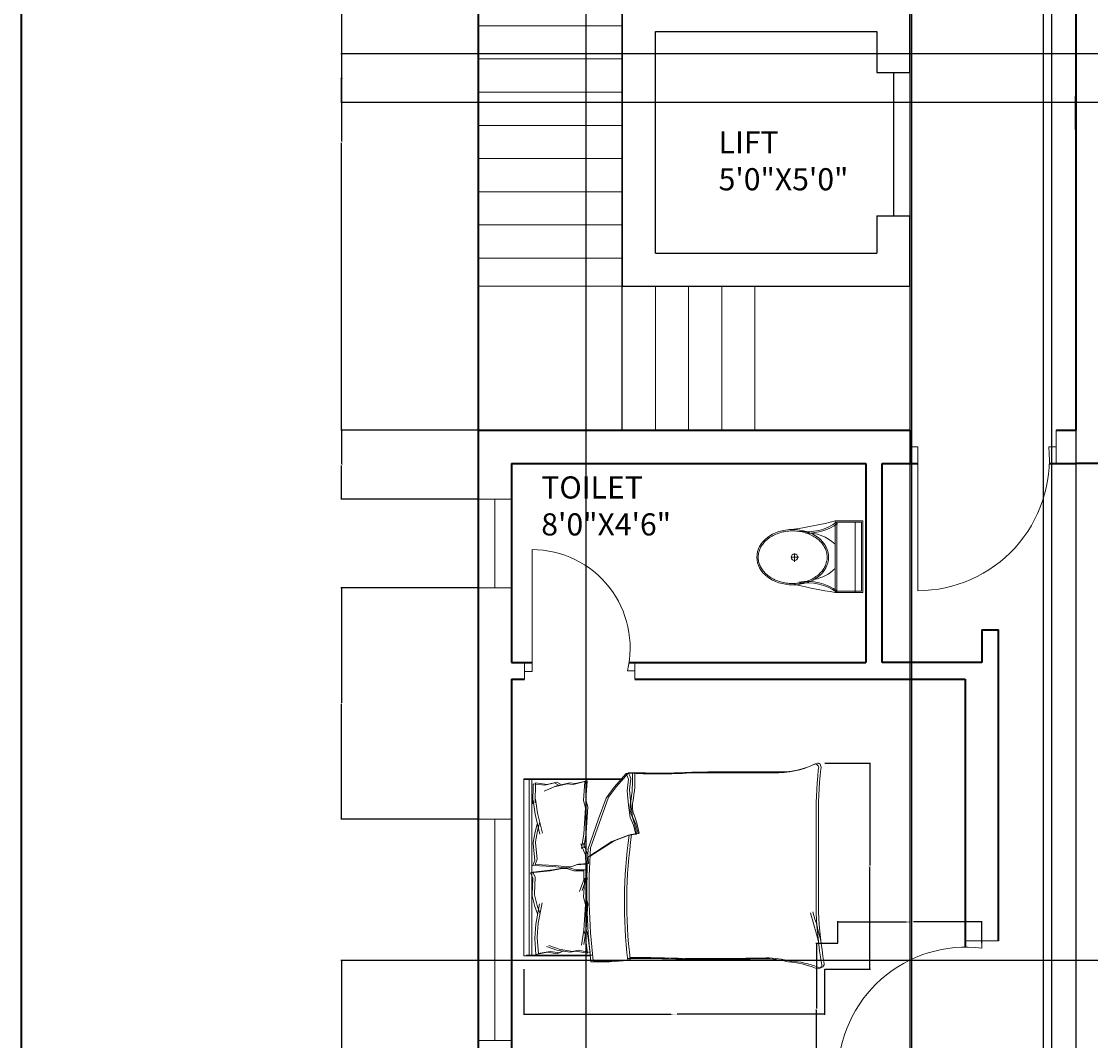
# Model space of a CAD drawing. Units: inches. Extents: x 1854 to 2495, y 1460 to 2772.
# Tile 2 of 12: x 1854 to 2144, y 1682 to 1958. Entities that reach past the tile are written whole.
import ezdxf

# ---------------------------------------------------------------- set-up
doc = ezdxf.new("R2010")
doc.units = ezdxf.units.IN
for name, color, linetype, lineweight in [('A-ANNO-DIMS', 2, 'Continuous', 18), ('A-ANNO-TTLB', 7, 'Continuous', 35), ('A-AREA-IDEN', 7, 'Continuous', 18), ('A-DOOR', 3, 'Continuous', 18), ('A-EQPM-ELEV', 7, 'Continuous', 25), ('A-FLOR-FIXT', 9, 'Continuous', 18), ('A-FLOR-STRS', 7, 'Continuous', 18), ('A-FURN', 8, 'Continuous', 13), ('A-GLAZ', 4, 'Continuous', 18), ('A-WALL', 7, 'Continuous', 35)]:
    doc.layers.add(name, color=color, linetype=linetype, lineweight=lineweight)
doc.styles.get("Standard").update_dxf_attribs({"font": 'arial.ttf'})
doc.dimstyles.get("Standard").update_dxf_attribs({"dimtxt": 0.18, "dimasz": 0.18, "dimexe": 0.18, "dimexo": 0.0625, "dimgap": 0.09, "dimtad": 0, "dimtih": 1, "dimtoh": 1, "dimdec": 4, "dimzin": 0, "dimdsep": 46, "dimtxsty": 'Standard', "dimcen": 0.09, "dimadec": 0, "dimazin": 0, "dimtfac": 1, "dimtdec": 4, "dimtofl": 0, "dimtmove": 0, "dimatfit": 3, "dimfxl": 1, "dimtolj": 1, "dimtzin": 0, "dimarcsym": 0})

# ---------------------------------------------------------------- blocks, each defined once
blk = doc.blocks.new('A$C31115884')
for p, q in [((283.1, 497.7), (223.4, 497.7)), ((257.5, 466.4), (257.5, 523.2)), ((0, 200), (0, 0)), ((520, 200), (0, 200)), ((10, 190), (10, 10)), ((510, 190), (10, 190)), ((510, 10), (510, 190)), ((520, 0), (520, 200)), ((510, 54.5), (0, 54.5)), ((10, 10), (510, 10)), ((0, 0), (520, 0))]:
    blk.add_line(p, q)
blk.add_circle((255.6, 496.4), 23.6)
for centre, radius, start, end in [((2777.7, -204.6), 2807, 165.4549, 171.71327), ((3237, 905), 2807, 188.28673, 194.5451), ((-294.5, 403.3), 364.7, 324.20913, 9.34987), ((-294.5, 403.3), 374.7, 324.20913, 9.34987), ((139.5, 406.2), 293.5, 315.84364, 2.65635), ((805.8, 403.3), 374.7, 179.20365, 215.79087), ((805.8, 403.3), 364.7, 170.65013, 215.79087), ((383.6, 406.2), 293.5, 190.27735, 224.15636)]:
    blk.add_arc(centre, radius, start, end)
blk.add_ellipse((256.2, 509.9), major_axis=(0, -260.7), ratio=0.772727)
blk.add_open_spline([(256.2, 259.2), (263.1, 259.2), (270, 259.7), (287.8, 262.3), (298.7, 265.1), (319.9, 273.1), (330.2, 278.4), (350.1, 291.1), (359.7, 298.7), (377.7, 315.9), (386.2, 325.5), (401.7, 346.6), (408.8, 358.1), (421.3, 382.5), (426.8, 395.5), (435.9, 422.4), (439.5, 436.4), (444.8, 465.1), (446.5, 479.7), (447.9, 509.2), (447.6, 524), (445, 553.3), (442.7, 567.8), (436.3, 596), (432.1, 609.7), (421.9, 636), (416, 648.6), (402.5, 672.1), (395, 683), (378.6, 703), (369.8, 712.1), (351.1, 728), (341.3, 734.8), (320.9, 746.2), (310.4, 750.7), (288.9, 757.3), (278, 759.4), (256, 761), (245, 760.6), (223.1, 757.2), (212.3, 754.3), (191.1, 746.1), (180.8, 740.7), (160.9, 727.8), (151.4, 720.1), (133.5, 702.7), (125.1, 693), (109.6, 671.7), (102.6, 660.2), (90.2, 635.7), (84.9, 622.7), (76, 595.6), (72.4, 581.6), (67.2, 552.9), (65.6, 538.2), (64.4, 508.8), (64.8, 494), (67.5, 464.7), (69.9, 450.2), (76.6, 422), (80.8, 408.3), (91.1, 382.2), (97.2, 369.7), (110.8, 346.3), (118.4, 335.4), (134.8, 315.6), (143.7, 306.7), (162.4, 290.9), (172.3, 284.2), (192.8, 273), (203.3, 268.6), (224.8, 262.2), (235.8, 260.2), (249.9, 259.3), (253, 259.2), (256.2, 259.2)], degree=3, knots=[0, 0, 0, 0, 0.110105, 0.110105, 0.285049, 0.285049, 0.459994, 0.459994, 0.634938, 0.634938, 0.809882, 0.809882, 0.984827, 0.984827, 1.159771, 1.159771, 1.334715, 1.334715, 1.50966, 1.50966, 1.684604, 1.684604, 1.859549, 1.859549, 2.034493, 2.034493, 2.209437, 2.209437, 2.384382, 2.384382, 2.559326, 2.559326, 2.73427, 2.73427, 2.909215, 2.909215, 3.084159, 3.084159, 3.259103, 3.259103, 3.434048, 3.434048, 3.608992, 3.608992, 3.783936, 3.783936, 3.958881, 3.958881, 4.133825, 4.133825, 4.30877, 4.30877, 4.483714, 4.483714, 4.658658, 4.658658, 4.833603, 4.833603, 5.008547, 5.008547, 5.183491, 5.183491, 5.358436, 5.358436, 5.53338, 5.53338, 5.708324, 5.708324, 5.883269, 5.883269, 6.058213, 6.058213, 6.233158, 6.233158, 6.283185, 6.283185, 6.283185, 6.283185])
blk = doc.blocks.new('BED-DOUBLE')
for p, q in [((27.75, 52.87), (24.5, 49.16)), ((27.75, 52.87), (24.5, 49.16)), ((28.39, 53.1), (25.14, 49.39)), ((28.39, 53.1), (25.14, 49.39)), ((29.49, 52.95), (27.75, 52.87, 3.87)), ((29.49, 52.95), (27.75, 52.87, 3.87)), ((28.37, 51.33), (27.75, 52.87)), ((28.37, 51.33), (27.75, 52.87)), ((30.13, 53.18), (28.39, 53.1, 3.87)), ((30.13, 53.18), (28.39, 53.1, 3.87)), ((29, 51.56), (28.39, 53.1)), ((29, 51.56), (28.39, 53.1)), ((0, 51.27), (0, 51.49)), ((0, 51.49), (0.64, 51.49)), ((0, 51.27), (26.61, 51.27)), ((0, 51.27), (26.61, 51.27)), ((0, 51.27), (0, 3.48)), ((0.64, 51.49), (27.25, 51.49)), ((0.64, 51.49), (27.25, 51.49)), ((1.53, 3.48), (1.53, 51.27)), ((1.53, 3.48), (1.53, 51.27)), ((2.17, 3.7), (2.17, 51.49)), ((2.17, 3.7), (2.17, 51.49)), ((2.56, 50.11), (2.46, 44.71)), ((2.56, 50.11), (2.46, 44.71)), ((2.56, 50.11), (5.77, 49.73)), ((2.56, 50.11), (5.77, 49.73)), ((3.2, 50.34), (3.1, 44.94)), ((3.2, 50.34), (3.1, 44.94)), ((3.2, 50.34), (6.41, 49.96)), ((3.2, 50.34), (6.41, 49.96)), ((8.26, 49.31), (5.58, 48.13)), ((8.26, 49.31), (5.58, 48.13)), ((5.77, 49.73), (8.34, 50.33)), ((5.77, 49.73), (8.34, 50.33)), ((8.9, 49.54), (6.22, 48.36)), ((8.9, 49.54), (6.22, 48.36)), ((6.41, 49.96), (8.98, 50.56)), ((6.41, 49.96), (8.98, 50.56)), ((11.83, 50.11), (8.26, 49.31)), ((11.83, 50.11), (8.26, 49.31)), ((8.34, 50.33), (9.38, 49.81)), ((8.34, 50.33), (9.38, 49.81)), ((12.47, 50.34), (8.9, 49.54)), ((12.47, 50.34), (8.9, 49.54)), ((8.98, 50.56), (10.02, 50.04)), ((8.98, 50.56), (10.02, 50.04)), ((13.43, 49.92), (11.83, 50.11)), ((13.43, 49.92), (11.83, 50.11)), ((14.07, 50.15), (12.47, 50.34)), ((14.07, 50.15), (12.47, 50.34)), ((16.57, 50.7), (13.43, 49.92)), ((16.57, 50.7), (13.43, 49.92)), ((17.21, 50.93), (14.07, 50.15)), ((17.21, 50.93), (14.07, 50.15)), ((16.17, 45.57), (16.57, 50.7)), ((16.17, 45.57), (16.57, 50.7)), ((16.81, 45.8), (17.21, 50.93)), ((16.81, 45.79), (17.21, 50.93)), ((25.14, 49.39), (22.97, 46.45)), ((25.14, 49.39), (22.97, 46.45)), ((28.06, 48.23), (28.37, 51.33)), ((28.06, 48.23), (28.37, 51.33)), ((28.7, 48.46), (29, 51.56)), ((28.7, 48.46), (29, 51.56)), ((22.97, 46.45), (20.96, 40.87)), ((22.97, 46.45), (20.96, 40.87)), ((24.5, 49.16), (22.33, 46.22)), ((24.5, 49.16), (22.33, 46.22)), ((28.37, 44.36), (28.06, 48.23)), ((28.37, 44.36), (28.06, 48.23)), ((29, 44.59), (28.7, 48.46)), ((29, 44.59), (28.7, 48.46)), ((2.46, 44.71), (2.54, 45.71)), ((2.46, 44.71), (2.54, 45.71)), ((2.54, 45.71), (3.07, 41.91)), ((2.54, 45.71), (3.07, 41.91)), ((3.1, 44.94), (3.18, 45.94)), ((3.1, 44.94), (3.18, 45.94)), ((3.18, 45.94), (3.71, 42.14)), ((3.18, 45.94), (3.71, 42.14)), ((16.73, 43.61), (16.17, 45.57)), ((16.73, 43.61), (16.17, 45.57)), ((16.3, 36.6), (16.73, 43.61)), ((16.3, 36.6), (16.73, 43.61)), ((17.37, 43.83), (16.81, 45.8)), ((17.37, 43.83), (16.81, 45.79)), ((16.93, 36.82), (17.37, 43.83)), ((16.93, 36.82), (17.37, 43.83)), ((22.33, 46.22), (20.32, 40.64)), ((22.33, 46.22), (20.32, 40.64)), ((28.83, 40.95), (28.37, 44.36)), ((28.83, 40.95), (28.37, 44.36)), ((29.47, 41.18), (29, 44.59)), ((29.47, 41.18), (29, 44.59)), ((3.07, 41.91), (4.42, 36.5)), ((3.07, 41.91), (4.42, 36.5)), ((3.71, 42.14), (5.06, 36.72)), ((3.71, 42.14), (5.06, 36.72)), ((20.32, 40.64), (17.38, 32.31)), ((20.32, 40.64), (17.38, 32.31)), ((20.96, 40.87), (18.02, 32.53)), ((20.96, 40.87), (18.02, 32.53)), ((29.76, 38.94), (28.83, 40.95)), ((29.76, 38.94), (28.83, 40.95)), ((30.4, 39.17), (29.47, 41.18)), ((30.4, 39.17), (29.47, 41.18)), ((3.67, 39.2), (3.08, 37.14)), ((3.67, 39.2), (3.08, 37.14)), ((4.31, 39.43), (3.72, 37.36)), ((4.31, 39.43), (3.72, 37.36)), ((30.38, 36.46), (29.76, 38.94)), ((30.38, 36.46), (29.76, 38.94)), ((31.02, 36.69), (30.4, 39.17)), ((31.02, 36.69), (30.4, 39.17)), ((79.25, 15.06), (79.25, 39.68)), ((79.25, 15.06), (79.25, 39.68)), ((79.88, 15.29), (79.88, 39.91)), ((79.88, 15.29), (79.88, 39.91)), ((3.08, 37.14), (2.54, 34.2)), ((3.08, 37.14), (2.54, 34.2)), ((3.72, 37.36), (3.18, 34.43)), ((3.72, 37.36), (3.18, 34.43)), ((15.63, 32.56), (16.3, 36.6)), ((15.63, 32.56), (16.3, 36.6)), ((16.27, 32.79), (16.93, 36.82)), ((16.27, 32.79), (16.93, 36.82)), ((23.88, 34.45), (28.37, 36.15)), ((23.88, 34.45), (28.37, 36.15)), ((24.52, 34.68), (29, 36.38)), ((24.52, 34.68), (29, 36.38)), ((28.37, 36.15), (30.38, 36.46)), ((28.37, 36.15), (30.38, 36.46)), ((29, 36.38), (31.02, 36.69)), ((29, 36.38), (31.02, 36.69)), ((2.54, 34.2), (2.56, 33.88)), ((2.54, 34.2), (2.56, 33.88)), ((2.56, 33.88), (2.98, 29.46)), ((2.56, 33.88), (2.98, 29.46)), ((3.18, 34.43), (3.2, 34.11)), ((3.18, 34.43), (3.2, 34.11)), ((3.2, 34.11), (3.62, 29.68)), ((3.2, 34.11), (3.62, 29.68)), ((16.74, 30.75), (15.45, 33.82)), ((16.74, 30.75), (15.45, 33.82)), ((17.38, 30.98), (16.09, 34.05)), ((17.38, 30.98), (16.09, 34.05)), ((17.38, 30.26), (23.88, 34.45)), ((17.38, 30.26), (23.88, 34.45)), ((18.02, 30.49), (24.52, 34.68)), ((18.02, 30.49), (24.52, 34.68)), ((2.98, 29.46), (2.49, 27.98)), ((2.98, 29.46), (2.49, 27.98)), ((3.62, 29.68), (3.13, 28.21)), ((3.62, 29.68), (3.13, 28.21)), ((16.89, 28.3), (16.74, 30.75)), ((16.89, 28.3), (16.74, 30.75)), ((17.53, 28.53), (17.38, 30.98)), ((17.53, 28.53), (17.38, 30.98)), ((1.87, 25.98), (7.22, 26.56)), ((1.87, 25.98), (7.22, 26.56)), ((2.49, 27.98), (7.87, 27.73)), ((2.49, 27.98), (7.87, 27.73)), ((2.51, 26.21), (7.86, 26.79)), ((2.51, 26.21), (7.86, 26.79)), ((3.09, 24.77), (2.51, 26.21)), ((3.09, 24.77), (2.51, 26.21)), ((3.13, 28.21), (8.51, 27.96)), ((3.13, 28.21), (8.51, 27.96)), ((7.22, 26.56), (10.4, 27.14)), ((7.22, 26.56), (10.4, 27.14)), ((7.86, 26.79), (11.04, 27.37)), ((7.86, 26.79), (11.04, 27.37)), ((7.87, 27.73), (11.08, 27.36)), ((7.87, 27.73), (11.08, 27.35)), ((8.51, 27.96), (11.72, 27.58)), ((8.51, 27.96), (11.72, 27.58)), ((10.4, 27.14), (11.7, 27.14)), ((10.4, 27.14), (11.7, 27.14)), ((11.04, 27.37), (12.34, 27.37)), ((11.04, 27.37), (12.34, 27.37)), ((11.08, 27.36), (12.38, 27.44)), ((11.08, 27.35), (12.38, 27.44)), ((11.7, 27.14), (13.58, 26.56)), ((11.7, 27.14), (13.58, 26.56)), ((11.72, 27.58), (13.02, 27.66)), ((11.72, 27.58), (13.02, 27.66)), ((12.34, 27.37), (14.22, 26.79)), ((12.34, 27.37), (14.22, 26.79)), ((12.38, 27.44), (14.22, 28.13)), ((12.38, 27.44), (14.22, 28.13)), ((13.02, 27.66), (14.86, 28.36)), ((13.02, 27.66), (14.86, 28.36)), ((13.58, 26.56), (16.26, 26.56)), ((13.58, 26.56), (16.26, 26.56)), ((14.22, 28.13), (16.89, 28.3)), ((14.22, 28.13), (16.89, 28.3)), ((14.22, 26.79), (16.9, 26.79)), ((14.22, 26.79), (16.9, 26.79)), ((14.86, 28.36), (17.53, 28.53)), ((14.86, 28.36), (17.53, 28.53)), ((16.26, 26.56), (16.26, 24.1)), ((16.26, 26.56), (16.26, 24.1)), ((16.9, 26.79), (16.9, 24.33)), ((16.9, 26.79), (16.9, 24.33)), ((2.45, 24.54), (1.87, 25.98)), ((2.45, 24.54), (1.87, 25.98)), ((2.3, 20.09), (2.45, 24.54)), ((2.3, 20.09), (2.45, 24.54)), ((2.94, 20.32), (3.09, 24.77)), ((2.94, 20.32), (3.09, 24.77)), ((16.26, 24.1), (15.17, 20.96)), ((16.26, 24.1), (15.17, 20.96)), ((16.9, 24.33), (15.81, 21.19)), ((16.9, 24.33), (15.81, 21.19)), ((16.17, 19.38), (16.57, 24.52)), ((16.17, 19.38), (16.57, 24.52)), ((16.81, 19.61), (17.21, 24.74)), ((16.81, 19.61), (17.21, 24.74)), ((2.94, 20), (2.94, 20.32)), ((2.94, 20), (2.94, 20.32)), ((2.3, 19.77), (2.3, 20.09)), ((2.3, 19.77), (2.3, 20.09)), ((3.03, 16.88), (2.3, 19.77)), ((3.03, 16.88), (2.3, 19.77)), ((3.67, 17.11), (2.94, 20)), ((3.67, 17.11), (2.94, 20)), ((3.32, 12.11), (4.33, 17.6)), ((3.32, 12.11), (4.33, 17.6)), ((3.96, 12.34), (4.97, 17.83)), ((3.96, 12.34), (4.97, 17.83)), ((16.73, 17.42), (16.17, 19.38)), ((16.73, 17.42), (16.17, 19.38)), ((16.3, 10.41), (16.73, 17.42)), ((16.3, 10.41), (16.73, 17.42)), ((17.37, 17.65), (16.81, 19.61)), ((17.37, 17.65), (16.81, 19.61)), ((16.93, 10.64), (17.37, 17.65)), ((16.93, 10.64), (17.37, 17.65)), ((3.75, 14.86), (3.03, 16.88)), ((3.75, 14.85), (3.03, 16.88)), ((4.39, 15.08), (3.67, 17.11)), ((4.39, 15.08), (3.67, 17.11)), ((3.03, 8.29), (3.32, 12.11)), ((3.03, 8.28), (3.32, 12.11)), ((3.67, 8.51), (3.96, 12.34)), ((3.67, 8.51), (3.96, 12.34)), ((15.63, 6.38), (16.3, 10.41)), ((15.63, 6.38), (16.3, 10.41)), ((16.27, 6.61), (16.93, 10.64)), ((16.27, 6.61), (16.93, 10.64)), ((16.3, 10.41), (16.62, 9.28)), ((16.3, 10.41), (16.62, 9.28)), ((16.62, 9.28), (17.34, 4.18)), ((16.62, 9.28), (17.34, 4.18)), ((16.93, 10.64), (17.26, 9.51)), ((16.93, 10.64), (17.26, 9.51)), ((17.26, 9.51), (17.98, 4.41)), ((17.26, 9.51), (17.98, 4.41)), ((3.01, 8.18), (3.03, 8.29)), ((3.01, 8.18), (3.03, 8.28)), ((3.34, 3.9), (3.01, 8.18)), ((3.34, 3.9), (3.01, 8.18)), ((3.65, 8.41), (3.67, 8.51)), ((3.65, 8.41), (3.67, 8.51)), ((3.98, 4.13), (3.65, 8.41)), ((3.98, 4.13), (3.65, 8.41)), ((8.96, 5.05), (6.21, 6.06)), ((8.96, 5.05), (6.21, 6.06)), ((9.59, 5.28), (6.85, 6.29)), ((9.59, 5.28), (6.85, 6.29)), ((18.11, 3.48), (0, 3.48)), ((18.11, 3.48), (0, 3.48)), ((18.75, 3.7), (0.64, 3.7)), ((18.75, 3.7), (0.64, 3.7)), ((3.32, 3.89), (6.5, 4.47)), ((3.32, 3.89), (6.5, 4.47)), ((3.96, 4.12), (7.14, 4.7)), ((3.96, 4.12), (7.14, 4.7)), ((6.5, 4.47), (9.1, 4.04)), ((6.5, 4.47), (9.1, 4.04)), ((7.14, 4.7), (9.74, 4.27)), ((7.14, 4.7), (9.74, 4.27)), ((12.57, 4.47), (8.96, 5.05)), ((12.57, 4.47), (8.96, 5.05)), ((9.1, 4.04), (10.11, 4.62)), ((9.1, 4.04), (10.11, 4.62)), ((13.21, 4.7), (9.59, 5.28)), ((13.21, 4.7), (9.59, 5.28)), ((9.74, 4.27), (10.75, 4.85)), ((9.74, 4.27), (10.75, 4.85)), ((14.16, 4.76), (12.57, 4.47)), ((14.16, 4.76), (12.57, 4.47)), ((14.8, 4.99), (13.21, 4.7)), ((14.8, 4.99), (13.21, 4.7)), ((17.34, 4.18), (14.16, 4.76)), ((17.34, 4.18), (14.16, 4.76)), ((17.98, 4.41), (14.8, 4.99)), ((17.98, 4.41), (14.8, 4.99))]:
    blk.add_line(p, q)
for centre, radius, start, end in [((68.67, 76.16), 23.07, 267.4714, 296.4681), ((68.67, 76.16), 23.07, 267.4714, 296.4681), ((69.31, 76.39), 23.07, 267.4714, 296.4681), ((69.31, 76.39), 23.07, 267.4714, 296.4681), ((78.87, 54.41), 1.1, 332.6588, 86.02), ((78.87, 54.41), 1.1, 332.6588, 86.02), ((79.51, 54.64), 1.1, 332.6588, 86.02), ((79.51, 54.64), 1.1, 332.6588, 86.02), ((-6.66, 51.33), 36.18, 349.8763, 2.5657), ((-6.66, 51.33), 36.18, 349.8763, 2.5657), ((36.32, 182.27), 129.5, 266.9791, 273.8365), ((36.32, 182.27), 129.5, 266.9791, 273.8365), ((-6.02, 51.56), 36.18, 349.8763, 2.5657), ((-6.02, 51.56), 36.18, 349.8763, 2.5657), ((36.95, 182.49), 129.5, 266.9791, 273.8365), ((36.95, 182.49), 129.5, 266.9791, 273.8365), ((67.82, -4508.74), 4561.86, 90.00217, 90.28689), ((67.82, -4508.74), 4561.86, 90.00217, 90.28689), ((68.46, -4508.51), 4561.86, 90.00217, 90.28689), ((68.46, -4508.52), 4561.86, 90.00217, 90.28689), ((212.28, 41.15), 133.04, 174.4998, 180.6351), ((212.28, 41.15), 133.04, 174.4998, 180.6351), ((212.92, 41.38), 133.04, 174.4998, 180.6351), ((212.92, 41.38), 133.04, 174.4998, 180.6351), ((35.07, 43.74), 6.22, 168.6608, 203.7384), ((35.07, 43.74), 6.22, 168.6608, 203.7384), ((35.71, 43.97), 6.22, 168.6608, 203.7384), ((35.71, 43.97), 6.22, 168.6608, 203.7384), ((1.48, 31.15), 29.65, 10.6617, 19.8806), ((1.48, 31.15), 29.65, 10.6617, 19.8806), ((2.12, 31.38), 29.65, 10.6617, 19.8806), ((2.12, 31.38), 29.65, 10.6617, 19.8806), ((156.32, 17.76), 129.02, 171.7845, 186.9006), ((156.32, 17.76), 129.02, 171.7845, 186.9006), ((156.96, 17.98), 129.02, 171.7845, 186.9006), ((156.96, 17.98), 129.02, 171.7845, 186.9006), ((30.44, 36.64), 0.185, 250.2464, 1.1377), ((30.44, 36.64), 0.185, 250.2464, 1.1377), ((31.08, 36.86), 0.185, 250.2464, 1.1377), ((31.08, 36.86), 0.185, 250.2464, 1.1377), ((182.05, 21.36), 164.97, 176.0865, 186.7821), ((182.05, 21.36), 164.97, 176.0865, 186.7821), ((182.69, 21.59), 164.97, 176.0865, 186.7821), ((182.69, 21.59), 164.97, 176.0865, 186.7821), ((-23.71, -17.22), 106.46, 13.3832, 17.7053), ((-23.71, -17.22), 106.46, 13.3832, 17.7053), ((-23.07, -16.99), 106.46, 13.3832, 17.7053), ((-23.07, -16.99), 106.46, 13.3832, 17.7053), ((200.84, 21.43), 121.76, 182.9958, 189.4091), ((200.84, 21.43), 121.76, 182.9958, 189.4091), ((201.48, 21.66), 121.76, 182.9958, 189.4091), ((201.48, 21.66), 121.76, 182.9958, 189.4091), ((31.81, -167.08), 170.11, 88.4762, 91.0082), ((31.81, -167.08), 170.11, 88.4762, 91.0082), ((51.25, 485.05), 482.31, 268.2277, 271.7185), ((51.25, 485.05), 482.31, 268.2277, 271.7185), ((65.15, -26.67), 29.63, 76.0648, 88.9113), ((65.15, -26.67), 29.63, 76.0648, 88.9113), ((20.1, 85.16), 83.31, 268.7218, 275.604), ((20.1, 85.16), 83.31, 268.7218, 275.604), ((20.74, 85.39), 83.31, 268.7218, 275.604), ((20.74, 85.39), 83.31, 268.7218, 275.604), ((31.17, -167.31), 170.11, 88.4762, 91.0082), ((31.17, -167.31), 170.11, 88.4762, 91.0082), ((50.61, 484.82), 482.31, 268.2277, 271.7185), ((50.61, 484.82), 482.31, 268.2277, 271.7185), ((64.52, -26.9), 29.63, 76.0648, 88.9113), ((64.52, -26.9), 29.63, 76.0648, 88.9113), ((70.28, -21.66), 23.56, 67.9751, 86.652), ((70.28, -21.66), 23.56, 67.9751, 86.652), ((70.92, -21.43), 23.56, 67.9751, 86.652), ((70.92, -21.43), 23.56, 67.9751, 86.652), ((79.72, 1.09), 1.09, 236.1736, 23.4781), ((79.72, 1.09), 1.09, 236.1736, 23.4781), ((80.36, 1.32), 1.09, 236.1736, 23.4781), ((80.36, 1.32), 1.09, 236.1736, 23.4781)]:
    blk.add_arc(centre, radius, start, end)
blk = doc.blocks.new('WINDOW-60IN')
for p, q in [((0, 9), (0, 0)), ((60, 4.5), (60, 9)), ((60, 9), (60, 0)), ((0, 0), (0, 4.5)), ((0, 4.5), (60, 4.5))]:
    blk.add_line(p, q)
blk = doc.blocks.new('DOOR-39IN-SWING')
blk.add_line((39, 0), (0, 0))
blk.add_arc((34.67, 0), 34.66, 82.8159, 180)
blk = doc.blocks.new('WINDOW-VENT-24IN')
for p, q in [((9, 24), (0, 24)), ((4.5, 24), (4.5, 0)), ((9, 0), (0, 0))]:
    blk.add_line(p, q)
blk = doc.blocks.new('*D21')
at = {"layer": 'A-ANNO-DIMS', "color": 0, "lineweight": -2, "transparency": 16777216}
for p, q in [((1990.3, 1700.95), (1990.3, 1688.6)), ((2071.85, 1700.95), (2071.85, 1688.6)), ((1990.48, 1688.78), (2030.26, 1688.78)), ((2071.67, 1688.78), (2031.89, 1688.78))]:
    blk.add_line(p, q, dxfattribs=at)
at = {"layer": 'A-ANNO-DIMS', "color": 0, "transparency": 16777216}
for points in [[(1990.48, 1688.81), (1990.48, 1688.75), (1990.3, 1688.78)], [(2071.67, 1688.81), (2071.67, 1688.75), (2071.85, 1688.78)]]:
    blk.add_solid(points, dxfattribs=at)
at = {"layer": 'Defpoints', "color": 0, "transparency": 16777216}
for p in [(1990.3, 1701.02), (2071.85, 1701.02), (2071.85, 1688.78)]:
    blk.add_point(p, dxfattribs=at)
at = {"layer": 'A-ANNO-DIMS', "color": 0, "transparency": 16777216, "insert": (2031.07, 1688.78), "char_height": 0.18, "attachment_point": 5}
blk.add_mtext('\\A1;BED 82 TYP.', dxfattribs=at)
blk = doc.blocks.new('*D22')
at = {"layer": 'A-ANNO-DIMS', "color": 0, "lineweight": -2, "transparency": 16777216}
for p, q in [((2071.91, 1756.84), (2084.26, 1756.84)), ((2084.08, 1756.66), (2084.08, 1729.11)), ((2084.08, 1701.2), (2084.08, 1728.75)), ((2071.91, 1701.02), (2084.26, 1701.02))]:
    blk.add_line(p, q, dxfattribs=at)
at = {"layer": 'A-ANNO-DIMS', "color": 0, "transparency": 16777216}
for points in [[(2084.05, 1756.66), (2084.11, 1756.66), (2084.08, 1756.84)], [(2084.05, 1701.2), (2084.11, 1701.2), (2084.08, 1701.02)]]:
    blk.add_solid(points, dxfattribs=at)
at = {"layer": 'Defpoints', "color": 0, "transparency": 16777216}
for p in [(2071.85, 1756.84), (2084.08, 1756.84), (2071.85, 1701.02)]:
    blk.add_point(p, dxfattribs=at)
at = {"layer": 'A-ANNO-DIMS', "color": 0, "transparency": 16777216, "insert": (2084.08, 1728.93), "char_height": 0.18, "attachment_point": 5}
blk.add_mtext('\\A1;56 TYP.', dxfattribs=at)
blk = doc.blocks.new('*D31')
at = {"layer": 'A-ANNO-DIMS', "color": 0, "lineweight": -2, "transparency": 16777216}
for p, q in [((2075.48, 1707.99), (2075.48, 1713.96)), ((2075.66, 1713.78), (2094.05, 1713.78)), ((2114.3, 1713.78), (2095.92, 1713.78)), ((2114.48, 1707.99), (2114.48, 1713.96))]:
    blk.add_line(p, q, dxfattribs=at)
at = {"layer": 'A-ANNO-DIMS', "color": 0, "transparency": 16777216}
for points in [[(2075.66, 1713.81), (2075.66, 1713.75), (2075.48, 1713.78)], [(2114.3, 1713.81), (2114.3, 1713.75), (2114.48, 1713.78)]]:
    blk.add_solid(points, dxfattribs=at)
at = {"layer": 'Defpoints', "color": 0, "transparency": 16777216}
for p in [(2114.48, 1713.78), (2075.48, 1707.93), (2114.48, 1707.93)]:
    blk.add_point(p, dxfattribs=at)
at = {"layer": 'A-ANNO-DIMS', "color": 0, "transparency": 16777216, "insert": (2094.98, 1713.78), "char_height": 0.18, "attachment_point": 5}
blk.add_mtext('\\A1;DOOR 39 TYP.', dxfattribs=at)
blk = doc.blocks.new('*D32')
at = {"layer": 'A-ANNO-DIMS', "color": 0, "lineweight": -2, "transparency": 16777216}
for p, q in [((2075.42, 1707.93), (2069.45, 1707.93)), ((2069.63, 1707.75), (2069.63, 1690.29)), ((2069.63, 1672.47), (2069.63, 1689.93)), ((2075.42, 1672.29), (2069.45, 1672.29))]:
    blk.add_line(p, q, dxfattribs=at)
at = {"layer": 'A-ANNO-DIMS', "color": 0, "transparency": 16777216}
for points in [[(2069.6, 1707.75), (2069.66, 1707.75), (2069.63, 1707.93)], [(2069.6, 1672.47), (2069.66, 1672.47), (2069.63, 1672.29)]]:
    blk.add_solid(points, dxfattribs=at)
at = {"layer": 'Defpoints', "color": 0, "transparency": 16777216}
for p in [(2069.63, 1707.93), (2075.48, 1707.93), (2075.48, 1672.29)]:
    blk.add_point(p, dxfattribs=at)
at = {"layer": 'A-ANNO-DIMS', "color": 0, "transparency": 16777216, "insert": (2069.63, 1690.11), "char_height": 0.18, "attachment_point": 5}
blk.add_mtext('\\A1;36 TYP.', dxfattribs=at)
blk = doc.blocks.new('*D50')
at = {"layer": 'A-ANNO-DIMS', "color": 0, "lineweight": -2, "transparency": 16777216}
for p, q in [((2381.04, 2272.04), (2418.21, 2272.04)), ((2418.03, 2271.86), (2418.03, 1933.48)), ((2418.03, 1594.72), (2418.03, 1933.11)), ((2119.04, 1594.54), (2418.21, 1594.54))]:
    blk.add_line(p, q, dxfattribs=at)
at = {"layer": 'A-ANNO-DIMS', "color": 0, "transparency": 16777216}
for points in [[(2418, 2271.86), (2418.06, 2271.86), (2418.03, 2272.04)], [(2418, 1594.72), (2418.06, 1594.72), (2418.03, 1594.54)]]:
    blk.add_solid(points, dxfattribs=at)
at = {"layer": 'Defpoints', "color": 0, "transparency": 16777216}
for p in [(2380.98, 2272.04), (2418.03, 2272.04), (2118.98, 1594.54)]:
    blk.add_point(p, dxfattribs=at)
at = {"layer": 'A-ANNO-DIMS', "color": 0, "transparency": 16777216, "insert": (2418.03, 1933.29), "char_height": 0.18, "attachment_point": 5}
blk.add_mtext('\\A1;677.5', dxfattribs=at)
blk = doc.blocks.new('*D52')
at = {"layer": 'A-ANNO-DIMS', "color": 0, "lineweight": -2, "transparency": 16777216}
for p, q in [((1977.92, 1804.3), (1940.75, 1804.3)), ((1940.93, 1804.12), (1940.93, 1773.15)), ((1940.93, 1741.81), (1940.93, 1772.78)), ((1977.92, 1741.63), (1940.75, 1741.63))]:
    blk.add_line(p, q, dxfattribs=at)
at = {"layer": 'A-ANNO-DIMS', "color": 0, "transparency": 16777216}
for points in [[(1940.9, 1804.12), (1940.96, 1804.12), (1940.93, 1804.3)], [(1940.9, 1741.81), (1940.96, 1741.81), (1940.93, 1741.63)]]:
    blk.add_solid(points, dxfattribs=at)
at = {"layer": 'Defpoints', "color": 0, "transparency": 16777216}
for p in [(1940.93, 1804.3), (1977.98, 1804.3), (1977.98, 1741.63)]:
    blk.add_point(p, dxfattribs=at)
at = {"layer": 'A-ANNO-DIMS', "color": 0, "transparency": 16777216, "insert": (1940.93, 1772.97), "char_height": 0.18, "attachment_point": 5}
blk.add_mtext('\\A1;62.68', dxfattribs=at)
blk = doc.blocks.new('*D53')
at = {"layer": 'A-ANNO-DIMS', "color": 0, "lineweight": -2, "transparency": 16777216}
for p, q in [((1977.92, 1847.04), (1940.75, 1847.04)), ((1940.93, 1846.86), (1940.93, 1837.86)), ((1940.93, 1828.48), (1940.93, 1837.49)), ((1977.92, 1828.3), (1940.75, 1828.3))]:
    blk.add_line(p, q, dxfattribs=at)
at = {"layer": 'A-ANNO-DIMS', "color": 0, "transparency": 16777216}
for points in [[(1940.9, 1846.86), (1940.96, 1846.86), (1940.93, 1847.04)], [(1940.9, 1828.48), (1940.96, 1828.48), (1940.93, 1828.3)]]:
    blk.add_solid(points, dxfattribs=at)
at = {"layer": 'Defpoints', "color": 0, "transparency": 16777216}
for p in [(1940.93, 1847.04), (1977.98, 1847.04), (1977.98, 1828.3)]:
    blk.add_point(p, dxfattribs=at)
at = {"layer": 'A-ANNO-DIMS', "color": 0, "transparency": 16777216, "insert": (1940.93, 1837.67), "char_height": 0.18, "attachment_point": 5}
blk.add_mtext('\\A1;18.74', dxfattribs=at)
blk = doc.blocks.new('*D54')
at = {"layer": 'A-ANNO-DIMS', "color": 0, "lineweight": -2, "transparency": 16777216}
for p, q in [((1977.92, 2003.04), (1940.75, 2003.04)), ((1940.93, 2002.86), (1940.93, 1925.23)), ((1940.93, 1847.22), (1940.93, 1924.86)), ((1977.92, 1847.04), (1940.75, 1847.04))]:
    blk.add_line(p, q, dxfattribs=at)
at = {"layer": 'A-ANNO-DIMS', "color": 0, "transparency": 16777216}
for points in [[(1940.9, 2002.86), (1940.96, 2002.86), (1940.93, 2003.04)], [(1940.9, 1847.22), (1940.96, 1847.22), (1940.93, 1847.04)]]:
    blk.add_solid(points, dxfattribs=at)
at = {"layer": 'Defpoints', "color": 0, "transparency": 16777216}
for p in [(1940.93, 2003.04), (1977.98, 2003.04), (1977.98, 1847.04)]:
    blk.add_point(p, dxfattribs=at)
at = {"layer": 'A-ANNO-DIMS', "color": 0, "transparency": 16777216, "insert": (1940.93, 1925.04), "char_height": 0.18, "attachment_point": 5}
blk.add_mtext('\\A1;156', dxfattribs=at)
blk = doc.blocks.new('*D61')
at = {"layer": 'A-ANNO-DIMS', "color": 0, "lineweight": -2, "transparency": 16777216}
for p, q in [((1977.98, 1847.11), (1977.98, 2309.27)), ((1978.16, 2309.09), (1997.26, 2309.09)), ((2016.8, 2309.09), (1997.7, 2309.09)), ((2016.98, 1847.11), (2016.98, 2309.27))]:
    blk.add_line(p, q, dxfattribs=at)
at = {"layer": 'A-ANNO-DIMS', "color": 0, "transparency": 16777216}
for points in [[(1978.16, 2309.12), (1978.16, 2309.06), (1977.98, 2309.09)], [(2016.8, 2309.12), (2016.8, 2309.06), (2016.98, 2309.09)]]:
    blk.add_solid(points, dxfattribs=at)
at = {"layer": 'Defpoints', "color": 0, "transparency": 16777216}
for p in [(2016.98, 2309.09), (1977.98, 1847.04), (2016.98, 1847.04)]:
    blk.add_point(p, dxfattribs=at)
at = {"layer": 'A-ANNO-DIMS', "color": 0, "transparency": 16777216, "insert": (1997.48, 2309.09), "char_height": 0.18, "attachment_point": 5}
blk.add_mtext('\\A1;39', dxfattribs=at)
blk = doc.blocks.new('*D62')
at = {"layer": 'A-ANNO-DIMS', "color": 0, "lineweight": -2, "transparency": 16777216}
for p, q in [((2139.98, 2002.98), (2139.98, 1503.44)), ((2094.98, 1963.98), (2094.98, 1503.44)), ((2095.16, 1503.62), (2117.26, 1503.62)), ((2139.8, 1503.62), (2117.71, 1503.62))]:
    blk.add_line(p, q, dxfattribs=at)
at = {"layer": 'A-ANNO-DIMS', "color": 0, "transparency": 16777216}
for points in [[(2095.16, 1503.65), (2095.16, 1503.59), (2094.98, 1503.62)], [(2139.8, 1503.65), (2139.8, 1503.59), (2139.98, 1503.62)]]:
    blk.add_solid(points, dxfattribs=at)
at = {"layer": 'Defpoints', "color": 0, "transparency": 16777216}
for p in [(2139.98, 2003.04), (2094.98, 1964.04), (2139.98, 1503.62)]:
    blk.add_point(p, dxfattribs=at)
at = {"layer": 'A-ANNO-DIMS', "color": 0, "transparency": 16777216, "insert": (2117.48, 1503.62), "char_height": 0.18, "attachment_point": 5}
blk.add_mtext('\\A1;45', dxfattribs=at)
blk = doc.blocks.new('*D63')
at = {"layer": 'A-ANNO-DIMS', "color": 0, "lineweight": -2, "transparency": 16777216}
for p, q in [((1977.98, 2246.39), (1977.98, 1503.44)), ((2007.19, 2246.48), (2007.19, 1503.44)), ((1978.16, 1503.62), (1992.21, 1503.62)), ((2007.01, 1503.62), (1992.96, 1503.62))]:
    blk.add_line(p, q, dxfattribs=at)
at = {"layer": 'A-ANNO-DIMS', "color": 0, "transparency": 16777216}
for points in [[(1978.16, 1503.65), (1978.16, 1503.59), (1977.98, 1503.62)], [(2007.01, 1503.65), (2007.01, 1503.59), (2007.19, 1503.62)]]:
    blk.add_solid(points, dxfattribs=at)
at = {"layer": 'Defpoints', "color": 0, "transparency": 16777216}
for p in [(1977.98, 2246.45), (2007.19, 2246.54), (2007.19, 1503.62)]:
    blk.add_point(p, dxfattribs=at)
at = {"layer": 'A-ANNO-DIMS', "color": 0, "transparency": 16777216, "insert": (1992.59, 1503.62), "char_height": 0.18, "attachment_point": 5}
blk.add_mtext('\\A1;29.21', dxfattribs=at)
blk = doc.blocks.new('*D66')
at = {"layer": 'A-ANNO-DIMS', "color": 0, "lineweight": -2, "transparency": 16777216}
for p, q in [((2371.92, 1703.31), (1940.75, 1703.31)), ((1940.93, 1703.13), (1940.93, 1673.86)), ((1940.93, 1644.22), (1940.93, 1673.5)), ((2371.92, 1644.04), (1940.75, 1644.04))]:
    blk.add_line(p, q, dxfattribs=at)
at = {"layer": 'A-ANNO-DIMS', "color": 0, "transparency": 16777216}
for points in [[(1940.9, 1703.13), (1940.96, 1703.13), (1940.93, 1703.31)], [(1940.9, 1644.22), (1940.96, 1644.22), (1940.93, 1644.04)]]:
    blk.add_solid(points, dxfattribs=at)
at = {"layer": 'Defpoints', "color": 0, "transparency": 16777216}
for p in [(1940.93, 1703.31), (2371.98, 1703.31), (2371.98, 1644.04)]:
    blk.add_point(p, dxfattribs=at)
at = {"layer": 'A-ANNO-DIMS', "color": 0, "transparency": 16777216, "insert": (1940.93, 1673.68), "char_height": 0.18, "attachment_point": 5}
blk.add_mtext('\\A1;59.27', dxfattribs=at)
blk = doc.blocks.new('*D67')
at = {"layer": 'A-ANNO-DIMS', "color": 0, "lineweight": -2, "transparency": 16777216}
for p, q in [((2371.92, 1949.04), (1940.75, 1949.04)), ((1940.93, 1948.86), (1940.93, 1942.6)), ((1940.93, 1935.97), (1940.93, 1942.24)), ((2371.92, 1935.79), (1940.75, 1935.79))]:
    blk.add_line(p, q, dxfattribs=at)
at = {"layer": 'A-ANNO-DIMS', "color": 0, "transparency": 16777216}
for points in [[(1940.9, 1948.86), (1940.96, 1948.86), (1940.93, 1949.04)], [(1940.9, 1935.97), (1940.96, 1935.97), (1940.93, 1935.79)]]:
    blk.add_solid(points, dxfattribs=at)
at = {"layer": 'Defpoints', "color": 0, "transparency": 16777216}
for p in [(1940.93, 1949.04), (2371.98, 1949.04), (2371.98, 1935.79)]:
    blk.add_point(p, dxfattribs=at)
at = {"layer": 'A-ANNO-DIMS', "color": 0, "transparency": 16777216, "insert": (1940.93, 1942.42), "char_height": 0.18, "attachment_point": 5}
blk.add_mtext('\\A1;13.252', dxfattribs=at)
blk = doc.blocks.new('*D71')
at = {"layer": 'A-ANNO-DIMS', "color": 0, "lineweight": -2, "transparency": 16777216}
for p, q in [((2095.37, 2002.98), (2095.37, 1503.44)), ((2133.34, 2002.98), (2133.34, 1503.44)), ((2095.55, 1503.62), (2113.96, 1503.62)), ((2133.16, 1503.62), (2114.75, 1503.62))]:
    blk.add_line(p, q, dxfattribs=at)
at = {"layer": 'A-ANNO-DIMS', "color": 0, "transparency": 16777216}
for points in [[(2095.55, 1503.65), (2095.55, 1503.59), (2095.37, 1503.62)], [(2133.16, 1503.65), (2133.16, 1503.59), (2133.34, 1503.62)]]:
    blk.add_solid(points, dxfattribs=at)
at = {"layer": 'Defpoints', "color": 0, "transparency": 16777216}
for p in [(2095.37, 2003.04), (2133.34, 2003.04), (2133.34, 1503.62)]:
    blk.add_point(p, dxfattribs=at)
at = {"layer": 'A-ANNO-DIMS', "color": 0, "transparency": 16777216, "insert": (2114.36, 1503.62), "char_height": 0.18, "attachment_point": 5}
blk.add_mtext('\\A1;37.97', dxfattribs=at)
blk = doc.blocks.new('*D73')
at = {"layer": 'A-ANNO-DIMS', "color": 0, "lineweight": -2, "transparency": 16777216}
for p, q in [((2131.08, 2220.98), (2131.08, 1503.44)), ((2216.32, 2220.98), (2216.32, 1503.44)), ((2131.26, 1503.62), (2173.31, 1503.62)), ((2216.14, 1503.62), (2174.1, 1503.62))]:
    blk.add_line(p, q, dxfattribs=at)
at = {"layer": 'A-ANNO-DIMS', "color": 0, "transparency": 16777216}
for points in [[(2131.26, 1503.65), (2131.26, 1503.59), (2131.08, 1503.62)], [(2216.14, 1503.65), (2216.14, 1503.59), (2216.32, 1503.62)]]:
    blk.add_solid(points, dxfattribs=at)
at = {"layer": 'Defpoints', "color": 0, "transparency": 16777216}
for p in [(2131.08, 2221.04), (2216.32, 2221.04), (2216.32, 1503.62)]:
    blk.add_point(p, dxfattribs=at)
at = {"layer": 'A-ANNO-DIMS', "color": 0, "transparency": 16777216, "insert": (2173.7, 1503.62), "char_height": 0.18, "attachment_point": 5}
blk.add_mtext('\\A1;85.25', dxfattribs=at)

msp = doc.modelspace()

# ---------------------------------------------------------------- linework, layer by layer
at = {"layer": 'A-ANNO-TTLB'}
msp.add_lwpolyline([(1854.1764, 2772.4852), (2494.521, 2772.4852), (2494.521, 1460.4076), (1854.1764, 1460.4076)], close=True, dxfattribs=at)
at = {"layer": 'A-DOOR'}
for p, q in [((2095.0976, 1838.0449), (2095.0976, 1847.0449)), ((2095.0976, 1847.0449), (2095.0976, 1842.5449)), ((2134.62, 1847.0449), (2134.62, 1838.0449)), ((2095.0976, 1842.5449), (2097.0976, 1842.5449)), ((2097.0976, 1842.5449), (2097.0976, 1803.5449)), ((2134.62, 1842.5449), (2132.62, 1842.5449)), ((2134.62, 1838.0449), (2134.62, 1842.5449)), ((1992.5652, 1781.6686), (1992.5652, 1814.6686)), ((1990.5652, 1784.0449), (1990.5652, 1780.3693)), ((2020.4007, 1784.0449), (2020.4007, 1779.5449)), ((1990.5652, 1779.5449), (1990.5652, 1781.6686)), ((1990.5652, 1781.6686), (1992.5652, 1781.6686)), ((1990.5652, 1780.3693), (1990.5652, 1779.5449)), ((2020.4007, 1781.7949), (2018.4007, 1781.7949)), ((2020.4007, 1779.5449), (2020.4007, 1781.7949)), ((2109.9824, 1708.6844), (2118.9824, 1708.6844)), ((2118.9824, 1708.6844), (2114.4824, 1708.6844)), ((2114.4824, 1708.6844), (2114.4824, 1706.6844))]:
    msp.add_line(p, q, dxfattribs=at)
for centre, radius, start, end in [((2097.0976, 1839.2224), 35.6774, 270, 5.343567), ((1992.5652, 1788.0797), 26.5889, 346.327684, 90)]:
    msp.add_arc(centre, radius, start, end, dxfattribs=at)
at = {"layer": 'A-EQPM-ELEV'}
for p, q in [((2016.9824, 1964.0449), (2016.9824, 1886.0449)), ((2094.9824, 1943.9813), (2094.9824, 1964.0449)), ((2025.9824, 1955.0449), (2085.9824, 1955.0449)), ((2025.9824, 1895.0449), (2025.9824, 1955.0449)), ((2085.9824, 1955.0449), (2085.9824, 1943.9813)), ((2085.9824, 1943.9813), (2085.9824, 1943.9813)), ((2085.9824, 1943.9813), (2094.9824, 1943.9813)), ((2090.4824, 1943.9813), (2090.4824, 1905.1523)), ((2085.9824, 1905.1523), (2094.9824, 1905.1523)), ((2085.9824, 1905.1523), (2085.9824, 1895.0449)), ((2094.9824, 1886.0449), (2094.9824, 1905.1523)), ((2025.9824, 1895.0449), (2085.9824, 1895.0449)), ((2016.9824, 1886.0449), (2094.9824, 1886.0449))]:
    msp.add_line(p, q, dxfattribs=at)
at = {"layer": 'A-FLOR-STRS'}
for p, q in [((2016.9824, 1956.6346), (1977.9824, 1956.6346)), ((2016.9824, 1947.6346), (1977.9824, 1947.6346)), ((2016.9824, 1938.6346), (1977.9824, 1938.6346)), ((2016.9824, 1929.6346), (1977.9824, 1929.6346)), ((2016.9824, 1920.6346), (1977.9824, 1920.6346)), ((2016.9824, 1911.6346), (1977.9824, 1911.6346)), ((2016.9824, 1902.6346), (1977.9824, 1902.6346)), ((2016.9824, 1893.6346), (1977.9824, 1893.6346)), ((2016.9824, 1886.0449), (1977.9824, 1886.0449)), ((2016.9824, 1886.0449), (2016.9824, 1847.0449)), ((2025.9824, 1886.0449), (2025.9824, 1847.0449)), ((2034.9824, 1886.0449), (2034.9824, 1847.0449)), ((2043.9824, 1886.0449), (2043.9824, 1847.0449)), ((2052.9824, 1886.0449), (2052.9824, 1847.0449))]:
    msp.add_line(p, q, dxfattribs=at)
at = {"layer": 'A-GLAZ'}
for p, q in [((1977.9824, 1828.3038), (1982.4824, 1828.3038)), ((1982.4824, 1804.3038), (1986.9824, 1804.3038))]:
    msp.add_line(p, q, dxfattribs=at)
at = {"layer": 'A-WALL'}
for p, q in [((1977.9824, 2202.5449), (1977.9824, 1594.5449)), ((2139.9824, 2003.0449), (2139.9824, 1847.0449)), ((2139.9824, 1928.5287), (2139.9824, 1937.5287)), ((1977.9824, 1847.0449), (2095.0976, 1847.0449)), ((2134.62, 1847.0449), (2139.9824, 1847.0449)), ((1986.9824, 1838.0449), (2082.9824, 1838.0449)), ((1986.9824, 1838.0449), (1986.9824, 1784.0449)), ((1986.9824, 1838.0449), (2082.9824, 1838.0449)), ((2082.9824, 1838.0449), (2082.9824, 1784.0449)), ((2087.4824, 1784.0449), (2087.4824, 1838.0449)), ((2087.4824, 1838.0449), (2097.0976, 1838.0449)), ((2132.7556, 1838.0449), (2139.9824, 1838.0449)), ((2148.9824, 1838.0449), (2139.9824, 1838.0449)), ((2114.4824, 1792.8965), (2114.4824, 1784.0449)), ((2114.4824, 1792.8965), (2118.9824, 1792.8965)), ((2118.9824, 1779.5449), (2118.9824, 1792.8965)), ((1986.9824, 1784.0449), (1992.5652, 1784.0449)), ((2018.8463, 1784.0449), (2082.9824, 1784.0449)), ((2114.4824, 1784.0449), (2087.4824, 1784.0449)), ((1986.9824, 1779.5449), (1990.5652, 1779.5449)), ((1986.9824, 1779.5449), (1986.9824, 1603.5449)), ((1986.9824, 1779.5449), (1990.5652, 1779.5449)), ((1986.9824, 1779.5449), (1986.9824, 1603.5449)), ((2020.4007, 1779.5449), (2087.4824, 1779.5449)), ((2020.4007, 1779.5449), (2109.9824, 1779.5449)), ((2109.9824, 1779.5449), (2109.9824, 1706.9562)), ((2118.9824, 1708.6844), (2118.9824, 1779.5449))]:
    msp.add_line(p, q, dxfattribs=at)

# ---------------------------------------------------------------- block references
at = {"layer": 'A-DOOR'}
msp.add_blockref('DOOR-39IN-SWING', (2075.482, 1672.292), dxfattribs=at)
at = {"layer": 'A-FLOR-FIXT', "xscale": 0.0372717239612423, "yscale": 0.0372717239612423, "zscale": 0.0372717239612423, "rotation": 89.99999999999999}
msp.add_blockref('A$C31115884', (2082.2108, 1803.0718), dxfattribs=at)
at = {"layer": 'A-FURN'}
msp.add_blockref('BED-DOUBLE', (1990.3002, 1701.1028), dxfattribs=at)
at = {"layer": 'A-GLAZ'}
msp.add_blockref('WINDOW-VENT-24IN', (1977.982, 1804.304), dxfattribs=at)
at = {"layer": 'A-GLAZ', "rotation": 270.0000000000002}
msp.add_blockref('WINDOW-60IN', (1977.9825, 1741.6269), dxfattribs=at)

# ---------------------------------------------------------------- texts
at = {"layer": 'A-AREA-IDEN', "char_height": 6, "attachment_point": 1}
for s, width, insert in [('LIFT\\P5\'0"X5\'0"', 105.854708, (2043.1277, 1928.0329)), ('TOILET\\P8\'0"X4\'6"', 79.953437, (1995.0655, 1834.5129))]:
    msp.add_mtext_dynamic_manual_height_columns(s, width=width, gutter_width=12.5, heights=[0], dxfattribs=dict(at, insert=insert))

# ---------------------------------------------------------------- dimensions: what is measured, and where the dimension line sits
at = {"layer": 'A-ANNO-DIMS'}
for base, p1, p2, override, picture, middle in [((2016.9824, 2309.0949), (1977.9824, 1847.0449), (2016.9824, 1847.0449), {"dimdec": 0, "dimlfac": 1, "dimrnd": 0, "dimzin": 0, "dimdsep": 46, "dimlunit": 2}, '*D61', (1997.4824, 2309.0949)), ((2007.1898, 1503.6207), (1977.9824, 2246.45), (2007.1898, 2246.5449), {"dimdec": 2, "dimlfac": 1, "dimrnd": 0, "dimzin": 0, "dimdsep": 46, "dimlunit": 2}, '*D63', (1992.5861, 1503.6207)), ((2216.3239, 1503.6207), (2131.0775, 2221.0449), (2216.3239, 2221.0449), {"dimdec": 2, "dimlfac": 1, "dimrnd": 0, "dimzin": 0, "dimdsep": 46, "dimlunit": 2}, '*D73', (2173.7007, 1503.6207)), ((2139.9824, 1503.6207), (2094.9824, 1964.0449), (2139.9824, 2003.0449), {"dimdec": 0, "dimlfac": 1, "dimrnd": 0, "dimzin": 0, "dimdsep": 46, "dimlunit": 2}, '*D62', (2117.4824, 1503.6207)), ((2133.341, 1503.6207), (2095.3698, 2003.0449), (2133.341, 2003.0449), {"dimdec": 2, "dimlfac": 1, "dimrnd": 0, "dimzin": 0, "dimdsep": 46, "dimlunit": 2}, '*D71', (2114.3554, 1503.6207))]:
    dim = msp.add_linear_dim(base=base, p1=p1, p2=p2, dimstyle='Standard', override=override, dxfattribs=at)
    dim.commit()
    dim.dimension.update_dxf_attribs({"geometry": picture, "text_midpoint": middle})
for base, p1, p2, override, picture, middle in [((2418.0324, 2272.0449), (2118.9824, 1594.5449), (2380.9824, 2272.0449), {"dimdec": 1, "dimlfac": 1, "dimrnd": 0, "dimzin": 0, "dimdsep": 46, "dimlunit": 2}, '*D50', (2418.0324, 1933.2949)), ((1940.9324, 2003.0449), (1977.9824, 1847.0449), (1977.9824, 2003.0449), {"dimdec": 0, "dimlfac": 1, "dimrnd": 0, "dimzin": 0, "dimdsep": 46, "dimlunit": 2}, '*D54', (1940.9324, 1925.0449)), ((1940.9324, 1949.0449), (2371.9824, 1935.7931), (2371.9824, 1949.0449), {"dimdec": 3, "dimlfac": 1, "dimrnd": 0, "dimzin": 0, "dimdsep": 46, "dimlunit": 2}, '*D67', (1940.9324, 1942.419)), ((1940.9324, 1847.0449), (1977.9824, 1828.3038), (1977.9824, 1847.0449), {"dimdec": 2, "dimlfac": 1, "dimrnd": 0, "dimzin": 0, "dimdsep": 46, "dimlunit": 2}, '*D53', (1940.9324, 1837.6744)), ((1940.9324, 1804.3038), (1977.9824, 1741.627), (1977.9824, 1804.3038), {"dimdec": 2, "dimlfac": 1, "dimrnd": 0, "dimzin": 0, "dimdsep": 46, "dimlunit": 2}, '*D52', (1940.9324, 1772.9654)), ((1940.9324, 1703.3147), (2371.9824, 1644.0449), (2371.9824, 1703.3147), {"dimdec": 2, "dimlfac": 1, "dimrnd": 0, "dimzin": 0, "dimdsep": 46, "dimlunit": 2}, '*D66', (1940.9324, 1673.6798))]:
    dim = msp.add_linear_dim(base=base, p1=p1, p2=p2, angle=90, dimstyle='Standard', override=override, dxfattribs=at)
    dim.commit()
    dim.dimension.update_dxf_attribs({"geometry": picture, "text_midpoint": middle})
for base, p1, p2, picture, middle in [((2084.0814, 1756.8411), (2071.8491, 1701.0166), (2071.8491, 1756.8411), '*D22', (2084.0814, 1728.9289)), ((2069.6324, 1707.9287), (2075.4824, 1672.2917), (2075.4824, 1707.9287), '*D32', (2069.6324, 1690.1102))]:
    dim = msp.add_linear_dim(base=base, p1=p1, p2=p2, angle=90, text='<> TYP.', dimstyle='Standard', override={"dimdec": 0, "dimlfac": 1, "dimrnd": 0, "dimzin": 0, "dimdsep": 46, "dimlunit": 2}, dxfattribs=at)
    dim.commit()
    dim.dimension.update_dxf_attribs({"geometry": picture, "text_midpoint": middle})
for base, p1, p2, text, picture, middle in [((2114.4824, 1713.7787), (2075.4824, 1707.9287), (2114.4824, 1707.9287), 'DOOR <> TYP.', '*D31', (2094.9824, 1713.7787)), ((2071.8491, 1688.7843), (1990.3005, 1701.0166), (2071.8491, 1701.0166), 'BED <> TYP.', '*D21', (2031.0748, 1688.7843))]:
    dim = msp.add_linear_dim(base=base, p1=p1, p2=p2, text=text, dimstyle='Standard', override={"dimdec": 0, "dimlfac": 1, "dimrnd": 0, "dimzin": 0, "dimdsep": 46, "dimlunit": 2}, dxfattribs=at)
    dim.commit()
    dim.dimension.update_dxf_attribs({"geometry": picture, "text_midpoint": middle})

doc.saveas('drawing.dxf')
